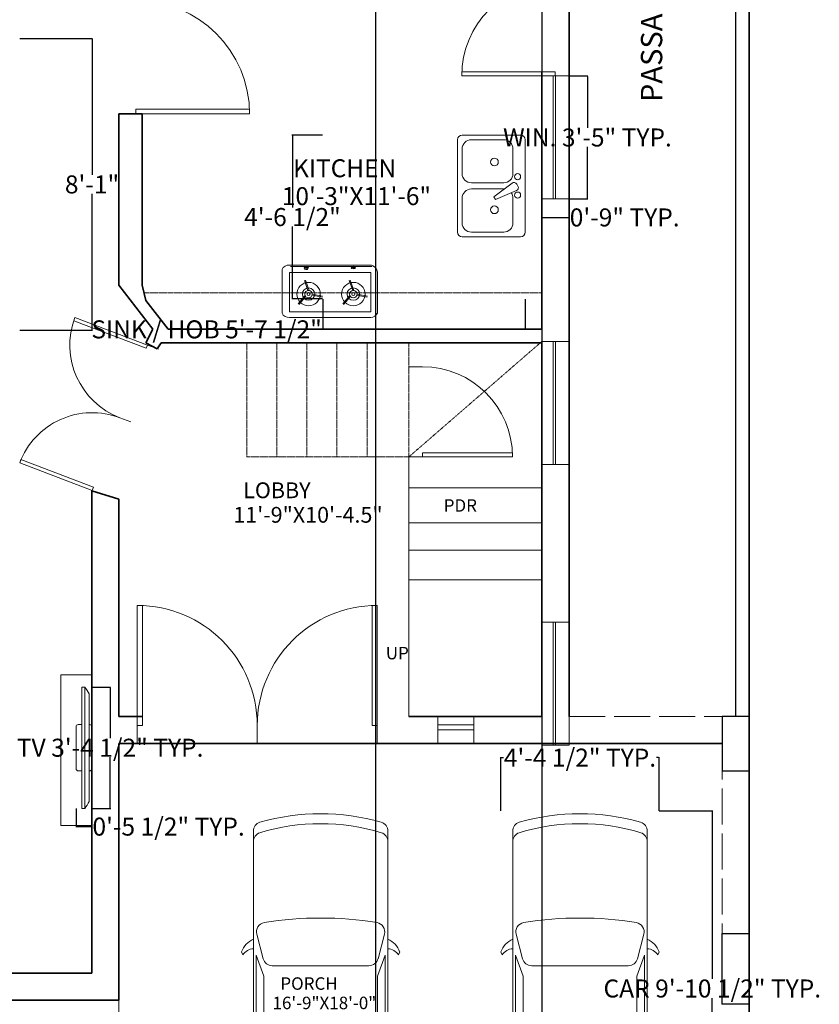
# Model space of a CAD drawing. Units: inches. Extents: x 79 to 8696167, y -3690578 to 147.
# Tile 3 of 10: x 310 to 577, y -551 to -223. Entities that reach past the tile are written whole.
import ezdxf

# ---------------------------------------------------------------- set-up
doc = ezdxf.new("R2010")
doc.units = ezdxf.units.IN
doc.header["$MEASUREMENT"] = 0
doc.linetypes.add('ACAD_ISO02W100', pattern=[15, 12, -3])
doc.linetypes.add('HIDDEN', pattern=[0.375, 0.25, -0.125])
doc.layers.get('0').update_dxf_attribs({"color": 253})
for name, color, linetype, lineweight in [('A-ANNO-DIMS', 2, 'Continuous', 18), ('A-AREA-IDEN', 7, 'Continuous', 18), ('A-DOOR', 4, 'Continuous', 18), ('A-EQPM', 9, 'Continuous', 18), ('A-FLOR-CASE-HIDN', 9, 'HIDDEN', 13), ('A-FLOR-PROJ', 8, 'ACAD_ISO02W100', 13), ('A-FLOR-STRS', 7, 'Continuous', 18), ('A-FLOR-STRS-OVHD', 8, 'HIDDEN', 13), ('C-PKNG-VEHI', 8, 'Continuous', 13), ('C-PROP', 7, 'Continuous', 35), ('C-SITE-WALL', 8, 'Continuous', 25), ('furniture', 30, 'Continuous', 18), ('garden', 114, 'Continuous', 18), ('PLUMBING FIXTURES', 9, 'Continuous', 18), ('text', 7, 'Continuous', 18), ('walls', 8, 'Continuous', 35), ('windows', 171, 'Continuous', 18)]:
    doc.layers.add(name, color=color, linetype=linetype, lineweight=lineweight)
doc.styles.add('ATT', font='TXT')
doc.styles.get("Standard").update_dxf_attribs({"font": 'arial.ttf'})
doc.dimstyles.get("Standard").update_dxf_attribs({"dimtxt": 6, "dimasz": 0.18, "dimexe": 0.18, "dimexo": 0.0625, "dimgap": 0.09, "dimtad": 0, "dimtih": 1, "dimtoh": 1, "dimzin": 0, "dimdsep": 46, "dimlunit": 3, "dimtxsty": 'Standard', "dimcen": 0.09, "dimadec": 0, "dimazin": 0, "dimtfac": 1, "dimtofl": 0, "dimtmove": 0, "dimatfit": 3, "dimfxl": 1, "dimtolj": 1, "dimtzin": 0, "dimarcsym": 0})

# ---------------------------------------------------------------- blocks, each defined once
blk = doc.blocks.new('15PSNK10')
at = {"color": 0, "linetype": 'ByBlock'}
for p, q in [((20.5, 16.5), (1.5, 16.5)), ((0, 15), (0, -15)), ((7, 15), (17.5, 15)), ((22, -15), (22, 15)), ((4, 4), (4, 12)), ((20.5, 12), (20.5, 4)), ((2.37, -0.1), (2.77, 0.6)), ((10.18, -3.57), (4.27, 0.87)), ((17.5, 1), (7, 1)), ((2.88, -1.54), (9.68, -4.43)), ((7.04, -1), (17.5, -1)), ((4, -12), (4, -4)), ((9.68, -4.43), (10.18, -3.57)), ((20.5, -4), (20.5, -12)), ((17.5, -15), (7, -15)), ((1.5, -16.5), (20.5, -16.5))]:
    blk.add_line(p, q, dxfattribs=at)
for centre, radius in [((10, 7.75), 1.25), ((2.5, 3), 1), ((2.5, -3), 1), ((10, -7.75), 1.25)]:
    blk.add_circle(centre, radius, dxfattribs=at)
for centre, radius, start, end in [((1.5, 15), 1.5, 90, 180), ((20.5, 15), 1.5, 0, 90), ((7, 12), 3, 90, 180), ((17.5, 12), 3, 0, 90), ((7, 4), 3, 180, 270), ((17.5, 4), 3, 270, 0), ((3.63, 0.1), 1, 50.5377, 150), ((3.23, -0.6), 1, 150, 249.4623), ((7, -4), 3, 146.607, 180), ((17.5, -4), 3, 0, 90), ((7, -12), 3, 180, 270), ((17.5, -12), 3, 270, 0), ((1.5, -15), 1.5, 180, 270), ((20.5, -15), 1.5, 270, 0)]:
    blk.add_arc(centre, radius, start, end, dxfattribs=at)
at = {"color": 0, "linetype": 'ByBlock', "style": 'ATT'}
for tag, p, flags in [('ITEM', (0, -26), 3), ('ROOM_NUMBER', (0, -35), 1)]:
    blk.add_attdef(tag, p, '', height=6, dxfattribs=dict(at, flags=flags))
blk = doc.blocks.new('PLASMA-LARGE')
at = {"layer": 'furniture'}
for p, q in [((-7.26, 0), (7.26, 0)), ((-21, -2.5), (21, -2.5)), ((-21, -2.5), (-21, -3.5)), ((-18.61, -1), (18.61, -1)), ((-8, -1), (-8, -0.74)), ((8, -1), (8, -0.74)), ((21, -2.5), (21, -3.5)), ((-21, -3.5), (21, -3.5)), ((-8, -3.5), (-8, -4.76)), ((-7.26, -5.5), (7.26, -5.5)), ((8, -3.5), (8, -4.76))]:
    blk.add_line(p, q, dxfattribs=at)
for centre, radius, start, end in [((-7.26, -0.74), 0.744, 90, 180), ((7.26, -0.74), 0.744, 0, 90), ((-13.97, -11.05), 11.07, 114.7602, 129.4175), ((13.97, -11.05), 11.07, 50.5825, 65.2398), ((-7.26, -4.76), 0.744, 180, 270), ((7.26, -4.76), 0.744, 270, 0)]:
    blk.add_arc(centre, radius, start, end, dxfattribs=at)
blk = doc.blocks.new('*U12')
for p, q in [((0, 0), (0, -6)), ((40, 0), (40, -6))]:
    blk.add_line(p, q)
blk.add_lwpolyline([(0, 0), (0, 40), (1.75, 40), (1.75, 0)], close=True)
blk.add_arc((0, 0), 40, 0, 90)
blk = doc.blocks.new('CAR')
at = {"layer": 'PLUMBING FIXTURES', "ltscale": 3}
for p, q in [((220804.47, -93720.06), (220804.47, -93547.3)), ((220876.86, -93720.06), (220876.86, -93547.35)), ((220870.5, -93584.17), (220875, -93575.44)), ((220810.83, -93584.17), (220806.31, -93577.76)), ((220810.23, -93596.08), (220805.58, -93585.68)), ((220805.58, -93585.68), (220805.58, -93603.85)), ((220871.11, -93596.08), (220875.75, -93585.68)), ((220875.75, -93585.68), (220875.75, -93603.85)), ((220810.23, -93603.85), (220810.23, -93596.08)), ((220871.11, -93603.85), (220871.11, -93596.08)), ((220805.58, -93603.85), (220810.23, -93603.85)), ((220875.75, -93603.85), (220871.11, -93603.85)), ((220805.99, -93608.09), (220810.13, -93608.09)), ((220805.99, -93653.29), (220805.99, -93608.09)), ((220810.13, -93608.09), (220810.13, -93642.08)), ((220875.35, -93608.09), (220871.21, -93608.09)), ((220871.21, -93608.09), (220871.21, -93642.08)), ((220875.35, -93653.29), (220875.35, -93608.09)), ((220810.13, -93642.08), (220805.99, -93653.29)), ((220871.21, -93642.08), (220875.35, -93653.29)), ((220806.3, -93664.61), (220809.78, -93651.39)), ((220814.66, -93647.63), (220866.67, -93647.63)), ((220875.03, -93664.61), (220871.56, -93651.39)), ((220798.82, -93653.49), (220798.11, -93655.1)), ((220882.52, -93653.49), (220883.22, -93655.1))]:
    blk.add_line(p, q, dxfattribs=at)
for centre, radius, start, end in [((220809.52, -93547.3), 5.05, 97.3566, 180), ((220840.49, -93811.75), 271.3, 83.2311, 96.6925), ((220840.49, -93815.88), 271.3, 83.2311, 96.6925), ((220871.81, -93547.35), 5.05, 360, 82.5593), ((220809.52, -93551.44), 5.05, 97.3566, 180), ((220871.81, -93551.49), 5.05, 360, 82.5593), ((220849.45, -93836.99), 262.8, 84.4202, 99.448), ((220840.67, -93184.08), 401.19, 265.7353, 274.2647), ((220814.66, -93652.68), 5.05, 90, 165.2564), ((220866.67, -93652.68), 5.05, 14.7436, 90), ((220809.44, -93651.03), 12.03, 199.7943, 245.6458), ((220804.88, -93649.65), 7.17, 212.3474, 266.7713), ((220876.46, -93649.65), 7.17, 273.2287, 327.6525), ((220871.9, -93651.03), 12.03, 294.3542, 340.2056), ((220811.18, -93665.89), 5.05, 165.2564, 260.0648), ((220870.15, -93665.89), 5.05, 279.9351, 14.7436), ((220840.67, -93484.81), 188.52, 260.7342, 279.2658), ((220809.52, -93714.44), 5.05, 180, 251.4636), ((220871.81, -93714.44), 5.05, 288.5363, 360), ((220809.52, -93720.06), 5.05, 180, 252.5507), ((220840.67, -93611.64), 112.45, 253.0675, 286.9325), ((220871.81, -93720.06), 5.05, 287.4493, 360), ((220840.67, -93610.47), 118.98, 254.0673, 285.9327)]:
    blk.add_arc(centre, radius, start, end, dxfattribs=at)
blk = doc.blocks.new('WIN-SIDE-41IN')
for p, q in [((0, 40.98), (9, 40.98)), ((0, 40.98), (0, 0)), ((3.73, 40.98), (3.73, 0)), ((4.5, 0), (4.5, 40.98)), ((9, 40.98), (9, 0)), ((9, 0), (0, 0))]:
    blk.add_line(p, q)
blk = doc.blocks.new('*D29')
at = {"layer": 'A-ANNO-DIMS', "color": 0, "lineweight": -2, "transparency": 16777216}
for p, q in [((493.5, -241.7), (499.77, -241.7)), ((499.59, -241.88), (499.59, -259.04)), ((499.59, -282.51), (499.59, -265.35)), ((493.5, -282.69), (499.77, -282.69))]:
    blk.add_line(p, q, dxfattribs=at)
at = {"layer": 'A-ANNO-DIMS', "color": 0, "lineweight": 100, "transparency": 16777216}
for points in [[(499.56, -241.88), (499.62, -241.88), (499.59, -241.7)], [(499.56, -282.51), (499.62, -282.51), (499.59, -282.69)]]:
    blk.add_solid(points, dxfattribs=at)
at = {"layer": 'Defpoints', "color": 0, "lineweight": 100, "transparency": 16777216}
for p in [(493.44, -241.7), (499.59, -241.7), (493.44, -282.69)]:
    blk.add_point(p, dxfattribs=at)
at = {"layer": 'A-ANNO-DIMS', "color": 0, "transparency": 16777216, "insert": (499.59, -262.2), "char_height": 6, "attachment_point": 5}
blk.add_mtext('\\A1;WIN. 3\'-5" TYP.', dxfattribs=at)
blk = doc.blocks.new('*D30')
at = {"layer": 'A-ANNO-DIMS', "color": 0, "lineweight": -2, "transparency": 16777216}
for p, q in [((484.44, -282.75), (484.44, -289.02)), ((493.44, -282.75), (493.44, -289.02)), ((484.62, -288.84), (493.26, -288.84)), ((493.44, -288.84), (493.62, -288.84))]:
    blk.add_line(p, q, dxfattribs=at)
at = {"layer": 'A-ANNO-DIMS', "color": 0, "lineweight": 100, "transparency": 16777216}
for points in [[(484.62, -288.81), (484.62, -288.87), (484.44, -288.84)], [(493.26, -288.81), (493.26, -288.87), (493.44, -288.84)]]:
    blk.add_solid(points, dxfattribs=at)
at = {"layer": 'Defpoints', "color": 0, "lineweight": 100, "transparency": 16777216}
for p in [(484.44, -282.69), (493.44, -282.69), (493.44, -288.84)]:
    blk.add_point(p, dxfattribs=at)
at = {"layer": 'A-ANNO-DIMS', "color": 0, "transparency": 16777216, "insert": (512, -288.84), "char_height": 6, "attachment_point": 5}
blk.add_mtext('\\A1;0\'-9" TYP.', dxfattribs=at)
blk = doc.blocks.new('*D39')
at = {"layer": 'A-ANNO-DIMS', "color": 0, "lineweight": -2, "transparency": 16777216}
for p, q in [((334.5, -445.33), (340.68, -445.33)), ((340.5, -445.51), (340.51, -462.36)), ((340.51, -485.59), (340.51, -468.75)), ((334.51, -485.77), (340.69, -485.77))]:
    blk.add_line(p, q, dxfattribs=at)
at = {"layer": 'A-ANNO-DIMS', "color": 0, "lineweight": 100, "transparency": 16777216}
for points in [[(340.53, -445.51), (340.47, -445.51), (340.5, -445.33)], [(340.54, -485.59), (340.48, -485.59), (340.51, -485.77)]]:
    blk.add_solid(points, dxfattribs=at)
at = {"layer": 'Defpoints', "color": 0, "lineweight": 100, "transparency": 16777216}
for p in [(334.44, -445.33), (340.5, -445.33), (334.44, -485.77)]:
    blk.add_point(p, dxfattribs=at)
at = {"layer": 'A-ANNO-DIMS', "color": 0, "transparency": 16777216, "insert": (340.51, -465.55), "char_height": 6, "attachment_point": 5}
blk.add_mtext('\\A1;TV 3\'-4 1/2" TYP.', dxfattribs=at)
blk = doc.blocks.new('*D40')
at = {"layer": 'A-ANNO-DIMS', "color": 0, "lineweight": -2, "transparency": 16777216}
for p, q in [((329.15, -485.83), (329.15, -492.02)), ((334.44, -485.83), (334.44, -492.02)), ((329.33, -491.84), (334.26, -491.84)), ((334.44, -491.84), (334.62, -491.84))]:
    blk.add_line(p, q, dxfattribs=at)
at = {"layer": 'A-ANNO-DIMS', "color": 0, "lineweight": 100, "transparency": 16777216}
for points in [[(329.33, -491.81), (329.33, -491.87), (329.15, -491.84)], [(334.26, -491.81), (334.26, -491.87), (334.44, -491.84)]]:
    blk.add_solid(points, dxfattribs=at)
at = {"layer": 'Defpoints', "color": 0, "lineweight": 100, "transparency": 16777216}
for p in [(329.15, -485.77), (334.44, -485.77), (334.44, -491.84)]:
    blk.add_point(p, dxfattribs=at)
at = {"layer": 'A-ANNO-DIMS', "color": 0, "transparency": 16777216, "insert": (359.99, -491.84), "char_height": 6, "attachment_point": 5}
blk.add_mtext('\\A1;0\'-5 1/2" TYP.', dxfattribs=at)
blk = doc.blocks.new('*D49')
at = {"layer": 'A-ANNO-DIMS', "color": 0, "lineweight": -2, "transparency": 16777216}
for p, q in [((411.39, -316.09), (411.39, -326.32)), ((478.87, -316.09), (478.87, -326.32)), ((411.39, -326.14), (411.21, -326.14)), ((478.69, -326.14), (411.57, -326.14))]:
    blk.add_line(p, q, dxfattribs=at)
at = {"layer": 'A-ANNO-DIMS', "color": 0, "lineweight": 100, "transparency": 16777216}
for points in [[(411.57, -326.11), (411.57, -326.17), (411.39, -326.14)], [(478.69, -326.11), (478.69, -326.17), (478.87, -326.14)]]:
    blk.add_solid(points, dxfattribs=at)
at = {"layer": 'Defpoints', "color": 0, "lineweight": 100, "transparency": 16777216}
for p in [(411.39, -316.02), (478.87, -316.02), (411.39, -326.14)]:
    blk.add_point(p, dxfattribs=at)
at = {"layer": 'A-ANNO-DIMS', "color": 0, "transparency": 16777216, "insert": (372.65, -326.14), "char_height": 6, "attachment_point": 5}
blk.add_mtext('\\A1;SINK / HOB 5\'-7 1/2"', dxfattribs=at)
blk = doc.blocks.new('*D50')
at = {"layer": 'A-ANNO-DIMS', "color": 0, "lineweight": -2, "transparency": 16777216}
for p, q in [((411.32, -261.4), (401.09, -261.4)), ((401.27, -261.58), (401.27, -285.52)), ((401.27, -315.84), (401.27, -291.9)), ((411.32, -316.02), (401.09, -316.02))]:
    blk.add_line(p, q, dxfattribs=at)
at = {"layer": 'A-ANNO-DIMS', "color": 0, "lineweight": 100, "transparency": 16777216}
for points in [[(401.24, -261.58), (401.3, -261.58), (401.27, -261.4)], [(401.24, -315.84), (401.3, -315.84), (401.27, -316.02)]]:
    blk.add_solid(points, dxfattribs=at)
at = {"layer": 'Defpoints', "color": 0, "lineweight": 100, "transparency": 16777216}
for p in [(401.27, -261.4), (411.39, -261.4), (411.39, -316.02)]:
    blk.add_point(p, dxfattribs=at)
at = {"layer": 'A-ANNO-DIMS', "color": 0, "transparency": 16777216, "insert": (401.27, -288.71), "char_height": 6, "attachment_point": 5}
blk.add_mtext('\\A1;4\'-6 1/2"', dxfattribs=at)
blk = doc.blocks.new('*D52')
at = {"layer": 'A-ANNO-DIMS', "color": 0, "lineweight": -2, "transparency": 16777216}
for p, q in [((310.42, -229.27), (334.65, -229.27)), ((334.47, -229.45), (334.47, -274.69)), ((334.47, -326.24), (334.47, -281)), ((310.42, -326.42), (334.65, -326.42))]:
    blk.add_line(p, q, dxfattribs=at)
at = {"layer": 'A-ANNO-DIMS', "color": 0, "lineweight": 100, "transparency": 16777216}
for points in [[(334.44, -229.45), (334.5, -229.45), (334.47, -229.27)], [(334.44, -326.24), (334.5, -326.24), (334.47, -326.42)]]:
    blk.add_solid(points, dxfattribs=at)
at = {"layer": 'Defpoints', "color": 0, "lineweight": 100, "transparency": 16777216}
for p in [(310.36, -229.27), (334.47, -229.27), (310.36, -326.42)]:
    blk.add_point(p, dxfattribs=at)
at = {"layer": 'A-ANNO-DIMS', "color": 0, "transparency": 16777216, "insert": (334.47, -277.84), "char_height": 6, "attachment_point": 5}
blk.add_mtext('\\A1;8\'-1"', dxfattribs=at)
blk = doc.blocks.new('*D53')
at = {"layer": 'A-ANNO-DIMS', "color": 0, "lineweight": -2, "transparency": 16777216}
for p, q in [((523.51, -486.61), (541.38, -486.61)), ((541.2, -486.79), (541.2, -542.6)), ((541.2, -604.78), (541.2, -548.98)), ((523.51, -604.96), (541.38, -604.96))]:
    blk.add_line(p, q, dxfattribs=at)
at = {"layer": 'A-ANNO-DIMS', "color": 0, "lineweight": 100, "transparency": 16777216}
for points in [[(541.17, -486.79), (541.23, -486.79), (541.2, -486.61)], [(541.17, -604.78), (541.23, -604.78), (541.2, -604.96)]]:
    blk.add_solid(points, dxfattribs=at)
at = {"layer": 'Defpoints', "color": 0, "lineweight": 100, "transparency": 16777216}
for p in [(523.45, -486.61), (523.45, -604.96), (541.2, -604.96)]:
    blk.add_point(p, dxfattribs=at)
at = {"layer": 'A-ANNO-DIMS', "color": 0, "transparency": 16777216, "insert": (541.2, -545.79), "char_height": 6, "attachment_point": 5}
blk.add_mtext('\\A1;CAR 9\'-10 1/2" TYP.', dxfattribs=at)
blk = doc.blocks.new('*D54')
at = {"layer": 'A-ANNO-DIMS', "color": 0, "lineweight": -2, "transparency": 16777216}
for p, q in [((470.75, -486.55), (470.75, -468.68)), ((470.93, -468.86), (471.61, -468.86)), ((523.27, -468.86), (522.59, -468.86)), ((523.45, -486.55), (523.45, -468.68))]:
    blk.add_line(p, q, dxfattribs=at)
at = {"layer": 'A-ANNO-DIMS', "color": 0, "lineweight": 100, "transparency": 16777216}
for points in [[(470.93, -468.83), (470.93, -468.89), (470.75, -468.86)], [(523.27, -468.83), (523.27, -468.89), (523.45, -468.86)]]:
    blk.add_solid(points, dxfattribs=at)
at = {"layer": 'Defpoints', "color": 0, "lineweight": 100, "transparency": 16777216}
for p in [(523.45, -468.86), (470.75, -486.61), (523.45, -486.61)]:
    blk.add_point(p, dxfattribs=at)
at = {"layer": 'A-ANNO-DIMS', "color": 0, "transparency": 16777216, "insert": (497.1, -468.86), "char_height": 6, "attachment_point": 5}
blk.add_mtext('\\A1;4\'-4 1/2" TYP.', dxfattribs=at)
blk = doc.blocks.new('*D57')
at = {"layer": 'A-ANNO-DIMS', "color": 0, "lineweight": -2, "transparency": 16777216}
for p, q in [((428.94, -155.06), (428.94, -723.2)), ((484.44, -155.06), (484.44, -723.2)), ((429.12, -723.02), (441.51, -723.02)), ((484.26, -723.02), (471.87, -723.02))]:
    blk.add_line(p, q, dxfattribs=at)
at = {"layer": 'A-ANNO-DIMS', "color": 0, "lineweight": 100, "transparency": 16777216}
for points in [[(429.12, -722.99), (429.12, -723.05), (428.94, -723.02)], [(484.26, -722.99), (484.26, -723.05), (484.44, -723.02)]]:
    blk.add_solid(points, dxfattribs=at)
at = {"layer": 'Defpoints', "color": 0, "lineweight": 100, "transparency": 16777216}
for p in [(428.94, -155), (484.44, -155), (484.44, -723.02)]:
    blk.add_point(p, dxfattribs=at)
at = {"layer": 'A-ANNO-DIMS', "color": 0, "transparency": 16777216, "insert": (456.69, -723.02), "char_height": 6, "attachment_point": 5}
blk.add_mtext('\\A1;4\'-7 1/2"', dxfattribs=at)

msp = doc.modelspace()

# ---------------------------------------------------------------- linework, layer by layer
at = {"layer": 'A-EQPM'}
for p, q in [((426.503, -304.761), (400.266, -304.761)), ((397.819, -320.703), (397.819, -306.167)), ((427.438, -307.155), (400.266, -307.155)), ((400.266, -307.155), (400.266, -320.295)), ((400.595, -305.142), (427.767, -305.142)), ((427.438, -320.295), (427.438, -307.155)), ((429.579, -320.777), (429.579, -307.155)), ((406.442, -313.179), (405.305, -309.859)), ((406.814, -313.174), (405.596, -309.772)), ((421.355, -313.179), (420.218, -309.859)), ((421.727, -313.174), (420.509, -309.772)), ((405.511, -314.847), (403.174, -317.603)), ((407.696, -314.712), (411.251, -315.358)), ((407.877, -314.387), (411.321, -315.063)), ((420.424, -314.847), (418.087, -317.603)), ((422.609, -314.712), (426.164, -315.358)), ((422.791, -314.387), (426.234, -315.063)), ((405.702, -315.167), (403.395, -317.812)), ((420.615, -315.167), (418.308, -317.812)), ((400.266, -320.295), (427.438, -320.295)), ((427.438, -322.18), (400.266, -322.18))]:
    msp.add_line(p, q, dxfattribs=at)
for centre, radius in [((406.646, -314.387), 3.912), ((421.559, -314.387), 3.912), ((406.646, -314.387), 2.08), ((406.646, -314.387), 1.225), ((406.646, -314.387), 0.507), ((421.559, -314.387), 2.08), ((421.559, -314.387), 1.225), ((421.559, -314.387), 0.507)]:
    msp.add_circle(centre, radius, dxfattribs=at)
for centre, radius, start, end in [((400.012, -307.151), 2.404, 83.93636, 156.89401), ((426.97, -307.334), 2.615, 3.92707, 100.30452), ((400.041, -319.786), 2.404, 202.40616, 275.36382), ((427.259, -319.571), 2.615, 273.92707, 332.5308)]:
    msp.add_arc(centre, radius, start, end, dxfattribs=at)
for centre, major_axis, ratio in [((421.563, -305.382), (0.713, -0.02), 0.3769734), ((405.785, -305.878), (0.664, -0.043), 0.4928397), ((405.893, -305.559), (0.713, -0.02), 0.3769734), ((421.555, -305.651), (0.664, -0.043), 0.4928397)]:
    msp.add_ellipse(centre, major_axis=major_axis, ratio=ratio, dxfattribs=at)
at = {"layer": 'A-FLOR-CASE-HIDN'}
msp.add_line((351.819, -313.966), (484.441, -313.966), dxfattribs=at)
at = {"layer": 'A-FLOR-PROJ'}
for p, q in [((493.441, -455.125), (553.441, -455.125)), ((544.441, -464.125), (544.441, -675.625))]:
    msp.add_line(p, q, dxfattribs=at)
at = {"layer": 'A-FLOR-STRS'}
for p, q in [((440.11, -330.625), (386.112, -330.625)), ((440.11, -368.606), (440.11, -455.125)), ((484.441, -378.952), (440.11, -378.952)), ((484.441, -390.648), (484.441, -378.952)), ((440.11, -399.759), (440.11, -390.648)), ((440.11, -390.648), (484.441, -390.648)), ((484.441, -399.759), (440.11, -399.759)), ((484.441, -409.554), (484.441, -399.759)), ((446.662, -409.554), (440.11, -409.554)), ((440.11, -409.554), (446.662, -409.554)), ((446.662, -409.554), (484.441, -409.554)), ((440.11, -455.125), (446.662, -455.125))]:
    msp.add_line(p, q, dxfattribs=at)
at = {"layer": 'A-FLOR-STRS-OVHD'}
for p, q in [((386.112, -330.625), (386.112, -368.606)), ((396.113, -330.625), (396.113, -368.606)), ((406.114, -330.625), (406.114, -368.606)), ((416.115, -330.625), (416.115, -368.606)), ((426.116, -330.625), (426.116, -368.606)), ((440.11, -368.606), (484.441, -330.139)), ((440.11, -368.606), (440.11, -330.625)), ((386.112, -368.606), (440.11, -368.606))]:
    msp.add_line(p, q, dxfattribs=at)
at = {"layer": 'C-PROP'}
msp.add_line((553.441, 99.875), (553.441, -680.125), dxfattribs=at)
at = {"layer": 'C-SITE-WALL'}
for p, q in [((548.941, 35.375), (548.941, -455.125)), ((544.441, -455.125), (544.441, -473.266)), ((553.441, -455.125), (544.441, -455.125)), ((553.441, -473.266), (553.441, -455.125)), ((544.441, -473.266), (553.441, -473.266)), ((544.441, -527.42), (553.441, -527.42)), ((544.441, -550.989), (544.441, -527.42)), ((553.441, -527.42), (553.441, -550.989)), ((553.441, -550.989), (544.441, -550.989))]:
    msp.add_line(p, q, dxfattribs=at)
at = {"layer": 'furniture'}
msp.add_lwpolyline([(324.071, -491.427), (324.067, -441.28), (334.439, -441.279), (334.443, -491.427)], close=True, dxfattribs=at)
at = {"layer": 'garden'}
msp.add_line((343.441, -549.625), (343.441, -680.125), dxfattribs=at)
at = {"layer": 'walls'}
for p, q in [((493.441, 35.375), (493.441, -455.125)), ((484.441, -240.344), (484.441, -326.125)), ((484.441, -240.344), (484.441, -326.125)), ((343.419, -269.483), (343.419, -254.372)), ((343.419, -254.372), (351.219, -254.372)), ((351.219, -254.372), (351.219, -311.407)), ((343.419, -269.483), (343.419, -311.407)), ((343.419, -311.407), (354.775, -326.125)), ((351.219, -311.407), (352.419, -316.524)), ((352.419, -316.524), (359.827, -326.125)), ((354.775, -326.125), (352.441, -330.625)), ((359.827, -326.125), (484.441, -326.125)), ((352.441, -330.625), (356.172, -332.597)), ((356.172, -332.597), (357.472, -330.625)), ((357.472, -330.625), (484.441, -330.625)), ((484.441, -330.625), (484.441, -455.125)), ((334.441, -540.625), (334.441, -379.75)), ((334.441, -379.991), (343.441, -382.739)), ((343.441, -455.125), (343.441, -382.739)), ((343.441, -455.125), (351.285, -455.125)), ((440.11, -455.125), (484.441, -455.125)), ((343.441, -549.625), (343.441, -464.125)), ((343.441, -464.125), (544.441, -464.125)), ((133.441, -540.625), (334.441, -540.625)), ((133.441, -549.625), (343.441, -549.625))]:
    msp.add_line(p, q, dxfattribs=at)
at = {"layer": 'windows'}
for p, q in [((449.745, -455.125), (449.745, -464.125)), ((461.727, -455.125), (449.745, -455.125)), ((449.745, -455.125), (449.745, -459.625)), ((461.727, -464.125), (461.727, -455.125)), ((461.727, -457.973), (449.745, -457.973)), ((461.727, -459.625), (461.727, -457.973)), ((449.745, -459.625), (461.727, -459.625)), ((449.745, -464.125), (461.727, -464.125))]:
    msp.add_line(p, q, dxfattribs=at)

# ---------------------------------------------------------------- block references
at = {"layer": 'A-DOOR'}
for p, xscale, yscale, zscale, rotation in [((488.775, -241.705), 0.7776860473082563, 0.7776860473082563, 0.7776860473082563, 90), ((349.103, -254.372), -0.9472671488816434, 0.9472671488816434, 0.9472671488816434, 270), ((352.962, -331.39), -0.6473174777509668, 0.6473174777509668, 0.6473174777509666, 69.19349462187056), ((444.609, -368.606), -0.7498099103642428, 0.7498099103642428, 0.7498099103642428, 270), ((334.567, -379.798), 0.6473174777509666, 0.6473174777509666, 0.6473174777509666, 69.19349462187061)]:
    msp.add_blockref('*U12', p, dxfattribs=dict(at, xscale=xscale, yscale=yscale, zscale=zscale, rotation=rotation))
msp.add_blockref('*U12', (349.535, -458.125), dxfattribs=at)
at = {"layer": 'A-DOOR', "xscale": -1}
msp.add_blockref('*U12', (429.535, -458.125), dxfattribs=at)
at = {"layer": 'C-PKNG-VEHI', "xscale": -0.6191396643141144, "yscale": 0.6191396643141144, "zscale": 0.6191396643141144, "rotation": 180}
for p in [(-136320.559, -58519.176), (-136234.115, -58519.176)]:
    msp.add_blockref('CAR', p, dxfattribs=at)
at = {"layer": 'furniture', "xscale": -0.9628364592350681, "yscale": 0.9628364592350692, "zscale": 0.9628364592350692, "rotation": 270.0090205836726}
msp.add_blockref('PLASMA-LARGE', (334.441, -465.552), dxfattribs=at)
at = {"layer": 'PLUMBING FIXTURES', "xscale": -1.026473487929304, "yscale": 1.026473487929304, "zscale": 1.026473487929304}
msp.add_blockref('15PSNK10', (478.866, -278.339), dxfattribs=at)
at = {"layer": 'windows'}
for p in [(484.441, -282.69), (484.441, -371.124), (484.441, -464.649)]:
    msp.add_blockref('WIN-SIDE-41IN', p, dxfattribs=at)

# ---------------------------------------------------------------- texts
at = {"layer": 'A-AREA-IDEN'}
msp.add_text('PASSAGE 5\'-0" WIDE', height=7.11297, rotation=90, dxfattribs=at).set_placement((524.516, -250.409))
for s, height, p in [('KITCHEN', 5.974, (401.477, -275.446)), ('10\'-3"X11\'-6"', 5.97402, (397.739, -284.73)), ('LOBBY', 5.26, (384.85, -382.394)), ('PDR', 4.1556, (451.678, -386.901)), ('11\'-9"X10\'-4.5"', 5.26001, (381.559, -390.569)), ('PORCH', 4.1556, (397.228, -546.221)), ('16\'-9"X18\'-0"', 4.15558, (394.627, -552.679))]:
    msp.add_text(s, height=height, dxfattribs=at).set_placement(p)
at = {"layer": 'text'}
msp.add_text('UP', height=4.1556, dxfattribs=at).set_placement((432.379, -436.102))

# ---------------------------------------------------------------- dimensions: what is measured, and where the dimension line sits
at = {"layer": 'A-ANNO-DIMS'}
dim = msp.add_linear_dim(base=(484.441, -723.025), p1=(428.941, -154.996), p2=(484.441, -154.996), dimstyle='Standard', override={"dimdec": 1, "dimlfac": 1, "dimrnd": 0, "dimzin": 1, "dimdsep": 46, "dimlunit": 4, "dimfrac": 2}, dxfattribs=at)
dim.commit()
dim.dimension.update_dxf_attribs({"geometry": '*D57', "text_midpoint": (456.691, -723.025)})
for base, p1, p2, picture, middle in [((334.468, -229.271), (310.359, -326.415), (310.359, -229.271), '*D52', (334.468, -277.843)), ((401.265, -261.402), (411.387, -316.023), (411.387, -261.402), '*D50', (401.265, -288.713))]:
    dim = msp.add_linear_dim(base=base, p1=p1, p2=p2, angle=90, dimstyle='Standard', override={"dimdec": 1, "dimlfac": 1, "dimrnd": 0, "dimzin": 1, "dimdsep": 46, "dimlunit": 4, "dimfrac": 2}, dxfattribs=at)
    dim.commit()
    dim.dimension.update_dxf_attribs({"geometry": picture, "text_midpoint": middle})
for base, p1, p2, angle, text, picture, middle in [((499.589, -241.705), (493.441, -282.69), (493.441, -241.705), 90, 'WIN. <> TYP.', '*D29', (499.589, -262.197)), ((411.387, -326.145), (478.866, -316.023), (411.387, -316.023), 180, 'SINK / HOB <>', '*D49', (372.645, -326.145)), ((340.503, -445.331), (334.444, -485.772), (334.438, -445.332), 90.00902, 'TV <> TYP.', '*D39', (340.507, -465.551)), ((334.445, -491.837), (329.148, -485.772), (334.444, -485.772), 0.00902, '<> TYP.', '*D40', (359.992, -491.837)), ((541.202, -604.964), (523.449, -486.613), (523.449, -604.964), 270, 'CAR <> TYP.', '*D53', (541.202, -545.788))]:
    dim = msp.add_linear_dim(base=base, p1=p1, p2=p2, angle=angle, text=text, dimstyle='Standard', override={"dimdec": 1, "dimlfac": 1, "dimrnd": 0, "dimzin": 1, "dimdsep": 46, "dimlunit": 4, "dimfrac": 2}, dxfattribs=at)
    dim.commit()
    dim.dimension.update_dxf_attribs({"geometry": picture, "text_midpoint": middle})
for base, p1, p2, picture, middle in [((493.441, -288.837), (484.441, -282.69), (493.441, -282.69), '*D30', (511.997, -288.837)), ((523.449, -468.86), (470.754, -486.613), (523.449, -486.613), '*D54', (497.101, -468.86))]:
    dim = msp.add_linear_dim(base=base, p1=p1, p2=p2, text='<> TYP.', dimstyle='Standard', override={"dimdec": 1, "dimlfac": 1, "dimrnd": 0, "dimzin": 1, "dimdsep": 46, "dimlunit": 4, "dimfrac": 2}, dxfattribs=at)
    dim.commit()
    dim.dimension.update_dxf_attribs({"geometry": picture, "text_midpoint": middle})

doc.saveas('drawing.dxf')
